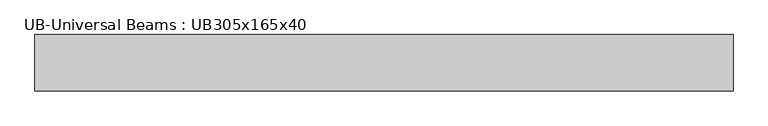
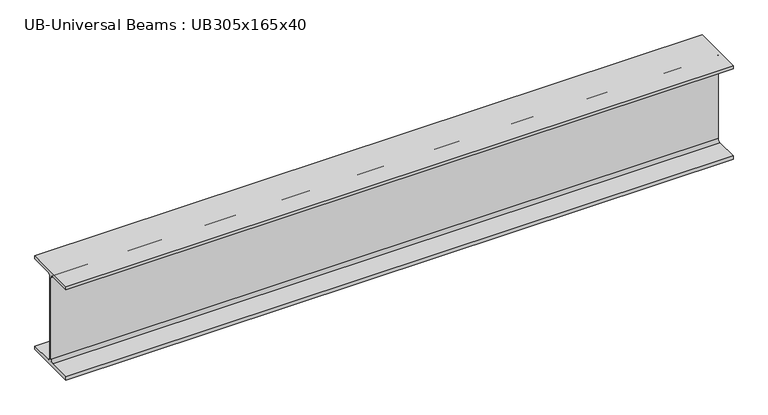
"""IFC4 building model written with IfcOpenShell, lengths in millimetres: beam geometry, UB-Universal Beams : UB305x165x40."""

from ifc_helpers import new_model, si_unit, point, frame, frame_2d, origin, place, context, project, spatial, polyline, circle_curve, trimmed, segment, composite_curve, outline, extrude, source, transform, mapped, element, save


def ub_universal_beams_ub305x165x40_d04475ed(model_context):
    return source(origin(), model_context, "Body", "SweptSolid", [
        extrude(outline(composite_curve([segment(polyline([(82.5, -141.5), (82.5, -151.7), (-82.5, -151.7), (-82.5, -141.5), (-11.9, -141.5)]), True, "CONTINUOUS"), segment(trimmed(circle_curve(frame_2d((-11.9, -132.6)), 8.9), [point((-11.9, -141.5))], [point((-3.0, -132.6))], True, "CARTESIAN"), True, "CONTINUOUS"), segment(polyline([(-3.0, -132.6), (-3.0, 132.6)]), True, "CONTINUOUS"), segment(trimmed(circle_curve(frame_2d((-11.9, 132.6)), 8.9), [point((-3.0, 132.6))], [point((-11.9, 141.5))], True, "CARTESIAN"), True, "CONTINUOUS"), segment(polyline([(-11.9, 141.5), (-82.5, 141.5), (-82.5, 151.7), (82.5, 151.7), (82.5, 141.5), (11.9, 141.5)]), True, "CONTINUOUS"), segment(trimmed(circle_curve(frame_2d((11.9, 132.6)), 8.9), [point((11.9, 141.5))], [point((3.0, 132.6))], True, "CARTESIAN"), True, "CONTINUOUS"), segment(polyline([(3.0, 132.6), (3.0, -132.6)]), True, "CONTINUOUS"), segment(trimmed(circle_curve(frame_2d((11.9, -132.6)), 8.9), [point((3.0, -132.6))], [point((11.9, -141.5))], True, "CARTESIAN"), True, "CONTINUOUS"), segment(polyline([(11.9, -141.5), (82.5, -141.5)]), True, "CONTINUOUS")], self_intersect=False)), frame((-1035.6, 0.0, 0.0), z_axis=(1.0, 0.0, 0.0), x_axis=(0.0, 1.0, 0.0)), (0.0, 0.0, 1.0), 2049.9),
    ])


if __name__ == "__main__":
    model = new_model("IFC4")
    model_context = context("Model", 3, world=origin())
    ifc_project = project(units=[si_unit("LENGTHUNIT", "METRE", prefix="MILLI")], contexts=[model_context])
    site = spatial("IfcSite", under=ifc_project)
    building = spatial("IfcBuilding", under=site)
    placement = place(None, origin())
    ub_universal_beams_ub305x165x40_shape = ub_universal_beams_ub305x165x40_d04475ed(model_context)
    element("IfcBeam", 1, ObjectType="UB-Universal Beams : UB305x165x40", at=placement, inside=building, context=model_context, shape_type="MappedRepresentation", body=[
        mapped(ub_universal_beams_ub305x165x40_shape, transform((0.0, 0.0, 0.0), x_axis=(1.0, 0.0, 0.0), y_axis=(0.0, 1.0, 0.0), z_axis=(0.0, 0.0, 1.0))),
    ])
    save(model, "model.ifc")

# Revit data of these elements
# Type "UB-Universal Beams : UB305x165x40"
#   Section Name Key = "UB305X165X40"
#   Width = 16.5 cm
#   Web Thickness = 0.6 cm
#   Web Fillet = 0.89 cm
#   Warping Constant = 164000.0 cm⁶
#   Torsional Moment of Inertia = 14.70 cm⁴
#   Section Area = 51.3 cm²
#   Plastic Modulus weak axis = 142.0 cm³
#   Plastic Modulus strong axis = 623.0 cm³
#   Nominal Weight = 40.2999 kgf/m
#   Moment of Inertia weak axis = 764.00 cm⁴
#   Moment of Inertia strong axis = 8503.00 cm⁴
#   Height = 30.34 cm
#   Flange Thickness = 1.02 cm
#   Elastic Modulus weak axis = 92.6 cm³
#   Elastic Modulus strong axis = 560.0 cm³
#   Centroid Vertical = 15.17 cm
#   Centroid Horizontal = 8.25 cm
#   Bolt Spacing = 9.0 cm
#   Length [instance default] = 1500 mm
#   Structural Material [instance default] = Metal - Steel 43-275
#   Type Comments = ""
#   Assembly Code = ""
# Element 1 (IfcBeam, "UB-Universal Beams : UB305x165x40")
#   Materials on its faces: "Metal - Steel 43-275"
# Materials
#   "Metal - Steel 43-275": class "Metal", colour RGB 247 247 247, transparency 0, Cost = 0
